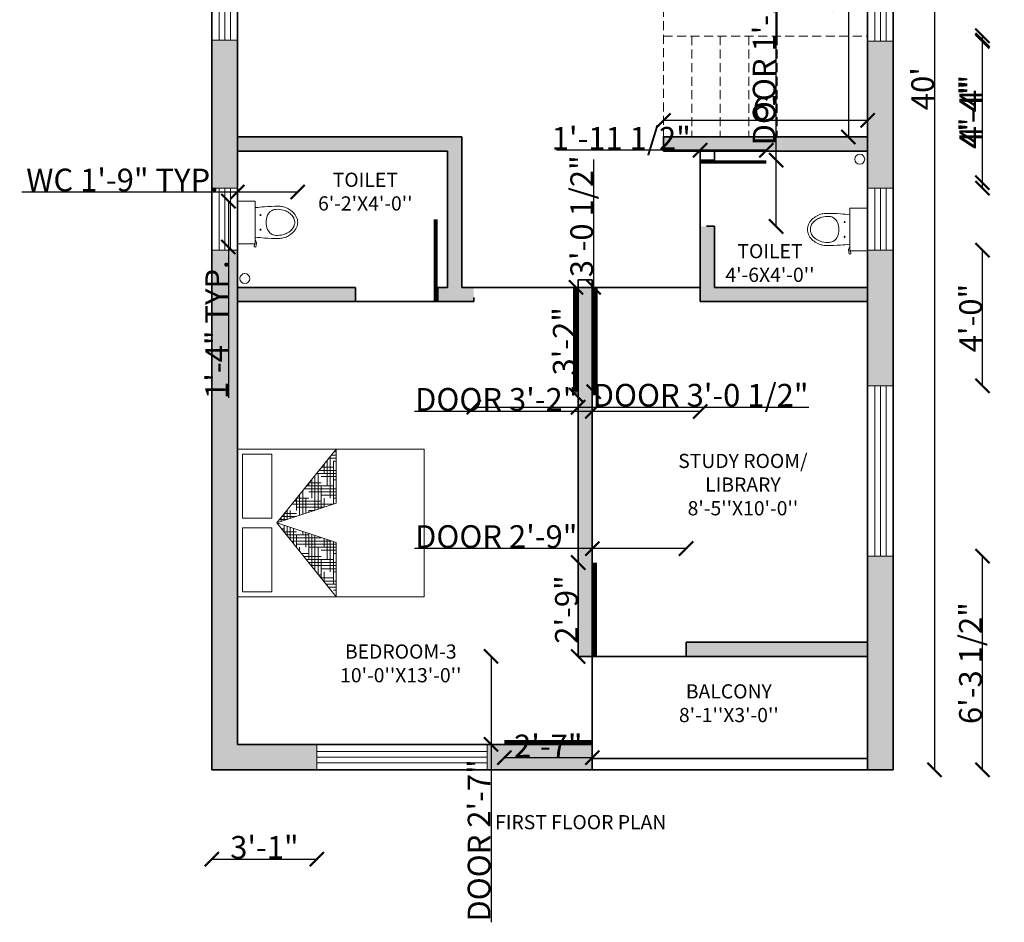
# Model space of a CAD drawing. Units: inches. Extents: x 2267 to 2908, y 1531 to 2136.
# Tile 4 of 5: x 2562 to 2908, y 1531 to 1849. Entities that reach past the tile are written whole.
import ezdxf

# ---------------------------------------------------------------- set-up
doc = ezdxf.new("R2010")
doc.units = ezdxf.units.IN
doc.linetypes.add('HIDDEN', pattern=[9.525, 6.35, -3.175])
for name, color, linetype, lineweight in [('A-ANNO-DIMS', 2, 'Continuous', 18), ('A-ANNO-TEXT', 7, 'Continuous', 18), ('A-AREA-IDEN', 7, 'Continuous', 18), ('A-FLOR-FIXT', 9, 'Continuous', 18), ('A-FLOR-STRS-HIDN', 50, 'HIDDEN', 13), ('A-FURN', 9, 'Continuous', 18), ('A-WALL-PATT', 8, 'Continuous', 13), ('DOOR', 30, 'Continuous', 18), ('STEPS', 50, 'Continuous', 18), ('WALL', 7, 'Continuous', 35), ('WINDOW', 152, 'Continuous', 18)]:
    doc.layers.add(name, color=color, linetype=linetype, lineweight=lineweight)
doc.styles.get("Standard").update_dxf_attribs({"font": 'arial.ttf'})
doc.dimstyles.get("Standard").update_dxf_attribs({"dimtxt": 8, "dimasz": 5, "dimexe": 0.18, "dimexo": 0.0625, "dimgap": 0.09, "dimtad": 1, "dimdec": 1, "dimzin": 0, "dimdsep": 46, "dimlunit": 4, "dimtxsty": 'Standard', "dimblk": 'ARCHTICK', "dimcen": 0.09, "dimse1": 1, "dimse2": 1, "dimadec": 0, "dimazin": 0, "dimtfac": 1, "dimtdec": 1, "dimtofl": 0, "dimtmove": 0, "dimatfit": 3, "dimfxl": 1, "dimtolj": 1, "dimtzin": 0, "dimarcsym": 0})

# ---------------------------------------------------------------- blocks, each defined once
blk = doc.blocks.new('A$C73484D89')
at = {"layer": 'DOOR'}
blk.add_lwpolyline([(1, 0, 0, 0, 0), (1, 0, 0, 0, 0), (0.975, 0, 0.05, 0.05, 0), (0.975, -1, 0, 0, 0), (0.95, -1, 0, 0, -0.429311), (0, 0, 0, 0, 0), (0, 0, 0, 0, 0)], format="xyseb", dxfattribs=at)
blk = doc.blocks.new('toilet-1')
at = {"color": 0, "linetype": 'ByBlock'}
for p, q in [((-0.23, -0.02), (-0.23, -0.212)), ((0.23, -0.02), (-0.23, -0.02)), ((0.23, -0.02), (0.23, -0.212)), ((-0.23, -0.212), (0.23, -0.212)), ((0.263, -0.2), (0.23, -0.204)), ((0.266, -0.219), (0.263, -0.2)), ((-0.089, -0.268), (-0.07, -0.268)), ((-0.079, -0.259), (-0.079, -0.278)), ((0.089, -0.268), (0.07, -0.268)), ((0.079, -0.259), (0.079, -0.278)), ((0.192, -0.214), (0.221, -0.225)), ((0.221, -0.225), (0.266, -0.219)), ((0, -0.638), (0, -0.638))]:
    blk.add_line(p, q, dxfattribs=at)
for centre, radius, start, end in [((1.737, -0.452), 1.911, 175.7698, 180.3758), ((3.527, -0.624), 3.709, 173.6925, 175.1593), ((-3.527, -0.624), 3.709, 4.8413, 6.3171), ((-1.737, -0.452), 1.911, 359.6242, 4.2302), ((-0.041, -0.44), 0.0996, 145.1497, 175.881), ((-0.031, -0.446), 0.111, 113.8997, 145.1485), ((0, -0.517), 0.188, 66.0939, 113.9061), ((0.031, -0.446), 0.111, 34.8515, 66.1003), ((0.041, -0.44), 0.0996, 4.119, 34.8503), ((0.035, -0.463), 0.209, 180.3747, 194.3375), ((0.055, -0.458), 0.23, 194.3353, 209.622), ((0.098, -0.45), 0.239, 175.8862, 195.5931), ((0.096, -0.45), 0.237, 195.5969, 209.3771), ((-0.096, -0.45), 0.237, 330.6229, 344.4031), ((-0.098, -0.45), 0.239, 344.4069, 4.1138), ((-0.055, -0.458), 0.23, 330.3788, 345.6655), ((-0.035, -0.463), 0.209, 345.6614, 359.6243), ((0.065, -0.452), 0.241, 209.6273, 224.5489), ((0.023, -0.491), 0.153, 209.3871, 226.5438), ((0.018, -0.499), 0.175, 224.552, 245.714), ((0.015, -0.5), 0.142, 226.5501, 246.5527), ((0, -0.535), 0.103, 246.5493, 270.0042), ((0, -0.535), 0.103, 269.9958, 293.4507), ((-0.015, -0.5), 0.142, 293.4473, 313.4499), ((-0.018, -0.499), 0.175, 294.2865, 315.4485), ((-0.023, -0.491), 0.153, 313.4562, 330.6129), ((-0.065, -0.452), 0.241, 315.4504, 330.372), ((0, -0.538), 0.132, 245.5845, 269.8782), ((0, -0.538), 0.132, 270.1216, 294.4153)]:
    blk.add_arc(centre, radius, start, end, dxfattribs=at)
blk = doc.blocks.new('*X6')
at = {"color": 0}
for p, q in [((20.156, 14.625), (20.156, 14.728)), ((20.174, 14.75), (20.277, 14.75)), ((20.188, 14.75), (20.188, 14.767)), ((20.199, 14.781), (20.277, 14.781)), ((20.25, 14.812), (20.277, 14.812)), ((20.25, 14.319), (20.25, 14.75)), ((20.094, 14.375), (20.094, 14.65)), ((20.098, 14.656), (20.125, 14.656)), ((20.124, 14.688), (20.25, 14.688)), ((20.125, 14.5), (20.125, 14.689)), ((20.149, 14.719), (20.277, 14.719)), ((19.998, 14.531), (20.277, 14.531)), ((20.023, 14.562), (20.277, 14.562)), ((20.031, 14.247), (20.031, 14.573)), ((20.062, 14.257), (20.062, 14.612)), ((20.125, 14.594), (20.277, 14.594)), ((20.219, 14.309), (20.219, 14.625)), ((20.25, 14.625), (20.277, 14.625)), ((19.922, 14.438), (20, 14.438)), ((19.948, 14.469), (20.125, 14.469)), ((19.973, 14.5), (20.25, 14.5)), ((20, 14.237), (20, 14.5)), ((20.188, 14.299), (20.188, 14.5)), ((20.25, 14.438), (20.277, 14.438)), ((19.844, 14.185), (19.844, 14.34)), ((19.875, 14.25), (19.875, 14.379)), ((19.875, 14.344), (20.277, 14.344)), ((19.906, 14.375), (19.906, 14.417)), ((19.969, 14.226), (19.969, 14.375)), ((20, 14.375), (20.277, 14.375)), ((20.125, 14.406), (20.277, 14.406)), ((20.156, 14.288), (20.156, 14.375)), ((19.772, 14.25), (20, 14.25)), ((19.781, 14.164), (19.781, 14.262)), ((19.797, 14.281), (20.125, 14.281)), ((19.812, 14.174), (19.812, 14.301)), ((19.822, 14.312), (20.229, 14.312)), ((19.938, 14.216), (19.938, 14.25)), ((19.721, 14.188), (19.75, 14.188)), ((19.746, 14.219), (19.875, 14.219)), ((19.75, 14.154), (19.75, 14.223)), ((19.702, 14.094), (19.779, 14.094)), ((19.719, 14.073), (19.719, 14.114)), ((19.727, 14.062), (19.873, 14.062)), ((19.75, 14.034), (19.75, 14.103)), ((19.752, 14.031), (19.875, 14.031)), ((19.781, 13.995), (19.781, 14.093)), ((19.812, 14), (19.812, 14.082)), ((19.906, 13.84), (19.906, 14.051)), ((19.938, 13.801), (19.938, 14.041)), ((19.969, 13.875), (19.969, 14.031)), ((19.827, 13.938), (20.25, 13.938)), ((19.875, 13.878), (19.875, 14)), ((19.875, 13.969), (20.156, 13.969)), ((20, 14), (20, 14.02)), ((20, 14), (20.061, 14)), ((20.062, 13.645), (20.062, 14)), ((20.094, 13.625), (20.094, 13.989)), ((20.125, 13.75), (20.125, 13.979)), ((20.156, 13.875), (20.156, 13.969)), ((20.25, 13.5), (20.25, 13.937)), ((19.853, 13.906), (20.125, 13.906)), ((19.878, 13.875), (20, 13.875)), ((20.031, 13.684), (20.031, 13.875)), ((20.125, 13.844), (20.277, 13.844)), ((20.219, 13.451), (20.219, 13.875)), ((20.25, 13.875), (20.277, 13.875)), ((19.953, 13.781), (20.277, 13.781)), ((19.978, 13.75), (20.25, 13.75)), ((20, 13.812), (20.277, 13.812)), ((20, 13.723), (20, 13.75)), ((20.188, 13.49), (20.188, 13.75)), ((20.003, 13.719), (20.125, 13.719)), ((20.125, 13.656), (20.277, 13.656)), ((20.25, 13.688), (20.277, 13.688)), ((20.079, 13.625), (20.277, 13.625)), ((20.104, 13.594), (20.277, 13.594)), ((20.129, 13.562), (20.25, 13.562)), ((20.156, 13.529), (20.156, 13.625)), ((20.205, 13.469), (20.277, 13.469)), ((20.23, 13.438), (20.277, 13.438)), ((20.25, 13.5), (20.277, 13.5)), ((20.255, 13.406), (20.277, 13.406))]:
    blk.add_line(p, q, dxfattribs=at)
blk = doc.blocks.new('MAT-P13')
for p, q in [((-0.75, 0), (0.75, 0)), ((-0.75, 0), (-0.75, -1.9)), ((0.75, 0), (0.75, -1.9)), ((-0.7, -0.05), (-0.7, -0.35)), ((-0.7, -0.05), (-0.05, -0.05)), ((-0.05, -0.35), (-0.05, -0.05)), ((0.05, -0.05), (0.7, -0.05)), ((0.05, -0.35), (0.05, -0.05)), ((0.7, -0.05), (0.7, -0.35)), ((-0.75, -1.003), (0, -0.4)), ((0, -0.4), (-0.75, -1.003)), ((-0.7, -0.35), (-0.05, -0.35)), ((0, -0.4), (-0.2, -1.003)), ((0, -0.4), (0.2, -1.003)), ((0, -0.4), (0.75, -1.003)), ((0.05, -0.35), (0.7, -0.35)), ((-0.75, -1.003), (-0.2, -1.003)), ((0.2, -1.003), (0.75, -1.003)), ((0.75, -1.9), (-0.75, -1.9))]:
    blk.add_line(p, q)
at = {"xscale": -1, "rotation": 90}
blk.add_blockref('*X6', (14.128, 19.274), dxfattribs=at)
blk = doc.blocks.new('_ArchTick')
at = {"color": 0, "linetype": 'ByBlock', "const_width": 0.15}
blk.add_lwpolyline([(-0.5, -0.5), (0.5, 0.5)], dxfattribs=at)
blk = doc.blocks.new('*D12')
at = {"layer": 'A-ANNO-DIMS', "color": 0, "lineweight": -2, "transparency": 16777216}
blk.add_line((2883.79, 2065.17), (2883.79, 1585.17), dxfattribs=at)
at = {"layer": 'Defpoints', "color": 0, "transparency": 16777216}
for p in [(2869.23, 2065.17), (2869.23, 1585.17), (2883.79, 1585.17)]:
    blk.add_point(p, dxfattribs=at)
at = {"layer": 'A-ANNO-DIMS', "color": 0, "lineweight": -2, "transparency": 16777216, "xscale": 5, "yscale": 5, "zscale": 5}
for p, rotation in [((2883.79, 2065.17), 90), ((2883.79, 1585.17), 270)]:
    blk.add_blockref('_ArchTick', p, dxfattribs=dict(at, rotation=rotation))
at = {"layer": 'A-ANNO-DIMS', "color": 0, "transparency": 16777216, "insert": (2879.62, 1825.17), "char_height": 8, "attachment_point": 5, "rotation": 90}
blk.add_mtext("\\A1;40'", dxfattribs=at)
blk = doc.blocks.new('*D14')
at = {"layer": 'A-ANNO-DIMS', "color": 0, "lineweight": -2, "transparency": 16777216}
blk.add_line((2853.44, 1919.17), (2853.44, 1808.17), dxfattribs=at)
at = {"layer": 'Defpoints', "color": 0, "transparency": 16777216}
for p in [(2860.23, 1919.17), (2853.44, 1808.17), (2860.23, 1808.17)]:
    blk.add_point(p, dxfattribs=at)
at = {"layer": 'A-ANNO-DIMS', "color": 0, "lineweight": -2, "transparency": 16777216, "xscale": 5, "yscale": 5, "zscale": 5}
for p, rotation in [((2853.44, 1919.17), 90), ((2853.44, 1808.17), 270)]:
    blk.add_blockref('_ArchTick', p, dxfattribs=dict(at, rotation=rotation))
at = {"layer": 'A-ANNO-DIMS', "color": 0, "transparency": 16777216, "insert": (2849.26, 1863.67), "char_height": 8, "attachment_point": 5, "rotation": 90}
blk.add_mtext('\\A1;9\'-3"', dxfattribs=at)
blk = doc.blocks.new('*D15')
at = {"layer": 'A-ANNO-DIMS', "color": 0, "lineweight": -2, "transparency": 16777216}
blk.add_line((2860.23, 1813.97), (2788.33, 1813.97), dxfattribs=at)
at = {"layer": 'Defpoints', "color": 0, "transparency": 16777216}
for p in [(2788.33, 1813.97), (2788.33, 1808.17), (2860.23, 1808.17)]:
    blk.add_point(p, dxfattribs=at)
at = {"layer": 'A-ANNO-DIMS', "color": 0, "lineweight": -2, "transparency": 16777216, "xscale": 5, "yscale": 5, "zscale": 5, "rotation": 180}
blk.add_blockref('_ArchTick', (2788.33, 1813.97), dxfattribs=at)
at = {"layer": 'A-ANNO-DIMS', "color": 0, "lineweight": -2, "transparency": 16777216, "xscale": 5, "yscale": 5, "zscale": 5}
blk.add_blockref('_ArchTick', (2860.23, 1813.97), dxfattribs=at)
at = {"layer": 'A-ANNO-DIMS', "color": 0, "transparency": 16777216, "insert": (2824.28, 1818.14), "char_height": 8, "attachment_point": 5}
blk.add_mtext("\\A1;6'", dxfattribs=at)
blk = doc.blocks.new('WIN-60IN')
for p, q in [((0, 6.5), (60, 6.5)), ((0, 4.5), (60, 4.5)), ((0, 2.5), (60, 2.5))]:
    blk.add_line(p, q)
blk.add_lwpolyline([(0, 9), (60, 9), (60, 0), (0, 0)], close=True)
blk = doc.blocks.new('WIN-43_65IN')
for p, q in [((2.5, 0), (2.5, 43.65)), ((4.5, 0), (4.5, 43.65)), ((6.5, 0), (6.5, 43.65))]:
    blk.add_line(p, q)
blk.add_lwpolyline([(0, 0), (0, 43.65), (9, 43.65), (9, 0)], close=True)
blk = doc.blocks.new('WIN-21_82IN')
for p, q in [((2.5, 0), (2.5, 21.82)), ((4.5, 0), (4.5, 21.82)), ((6.5, 0), (6.5, 21.82))]:
    blk.add_line(p, q)
blk.add_lwpolyline([(0, 0), (0, 21.82), (9, 21.82), (9, 0)], close=True)
blk = doc.blocks.new('*D29')
at = {"layer": 'A-ANNO-DIMS', "color": 0, "lineweight": -2, "transparency": 16777216}
for p, q in [((2763.23, 1711.47), (2700.55, 1711.47)), ((2801.24, 1711.47), (2763.23, 1711.47))]:
    blk.add_line(p, q, dxfattribs=at)
at = {"layer": 'Defpoints', "color": 0, "transparency": 16777216}
for p in [(2763.23, 1717.17), (2801.24, 1717.17), (2763.23, 1711.47)]:
    blk.add_point(p, dxfattribs=at)
at = {"layer": 'A-ANNO-DIMS', "color": 0, "lineweight": -2, "transparency": 16777216, "xscale": 5, "yscale": 5, "zscale": 5, "rotation": 180}
blk.add_blockref('_ArchTick', (2763.23, 1711.47), dxfattribs=at)
at = {"layer": 'A-ANNO-DIMS', "color": 0, "lineweight": -2, "transparency": 16777216, "xscale": 5, "yscale": 5, "zscale": 5}
blk.add_blockref('_ArchTick', (2801.24, 1711.47), dxfattribs=at)
at = {"layer": 'A-ANNO-DIMS', "color": 0, "transparency": 16777216, "insert": (2729.39, 1715.7), "char_height": 8, "attachment_point": 5}
blk.add_mtext('\\A1;DOOR 3\'-2"', dxfattribs=at)
blk = doc.blocks.new('*D30')
at = {"layer": 'A-ANNO-DIMS', "color": 0, "lineweight": -2, "transparency": 16777216}
blk.add_line((2757.53, 1717.17), (2757.53, 1755.17), dxfattribs=at)
at = {"layer": 'Defpoints', "color": 0, "transparency": 16777216}
for p in [(2757.53, 1755.17), (2763.23, 1755.17), (2763.23, 1717.17)]:
    blk.add_point(p, dxfattribs=at)
at = {"layer": 'A-ANNO-DIMS', "color": 0, "lineweight": -2, "transparency": 16777216, "xscale": 5, "yscale": 5, "zscale": 5}
for p, rotation in [((2757.53, 1755.17), 90), ((2757.53, 1717.17), 270)]:
    blk.add_blockref('_ArchTick', p, dxfattribs=dict(at, rotation=rotation))
at = {"layer": 'A-ANNO-DIMS', "color": 0, "transparency": 16777216, "insert": (2753.35, 1736.17), "char_height": 8, "attachment_point": 5, "rotation": 90}
blk.add_mtext('\\A1;3\'-2"', dxfattribs=at)
blk = doc.blocks.new('*D33')
at = {"layer": 'A-ANNO-DIMS', "color": 0, "lineweight": -2, "transparency": 16777216}
for p, q in [((2721.49, 1712.93), (2758.23, 1712.93)), ((2758.23, 1712.93), (2839.55, 1712.93))]:
    blk.add_line(p, q, dxfattribs=at)
at = {"layer": 'Defpoints', "color": 0, "transparency": 16777216}
for p in [(2721.49, 1718.44), (2758.23, 1718.44), (2758.23, 1712.93)]:
    blk.add_point(p, dxfattribs=at)
at = {"layer": 'A-ANNO-DIMS', "color": 0, "lineweight": -2, "transparency": 16777216, "xscale": 5, "yscale": 5, "zscale": 5, "rotation": 180}
blk.add_blockref('_ArchTick', (2721.49, 1712.93), dxfattribs=at)
at = {"layer": 'A-ANNO-DIMS', "color": 0, "lineweight": -2, "transparency": 16777216, "xscale": 5, "yscale": 5, "zscale": 5}
blk.add_blockref('_ArchTick', (2758.23, 1712.93), dxfattribs=at)
at = {"layer": 'A-ANNO-DIMS', "color": 0, "transparency": 16777216, "insert": (2801.39, 1717.16), "char_height": 8, "attachment_point": 5}
blk.add_mtext('\\A1;DOOR 3\'-0 1/2"', dxfattribs=at)
blk = doc.blocks.new('*D34')
at = {"layer": 'A-ANNO-DIMS', "color": 0, "lineweight": -2, "transparency": 16777216}
for p, q in [((2763.74, 1755.17), (2763.74, 1800.25)), ((2763.74, 1718.44), (2763.74, 1755.17))]:
    blk.add_line(p, q, dxfattribs=at)
at = {"layer": 'Defpoints', "color": 0, "transparency": 16777216}
for p in [(2758.23, 1755.17), (2763.74, 1755.17), (2758.23, 1718.44)]:
    blk.add_point(p, dxfattribs=at)
at = {"layer": 'A-ANNO-DIMS', "color": 0, "lineweight": -2, "transparency": 16777216, "xscale": 5, "yscale": 5, "zscale": 5}
for p, rotation in [((2763.74, 1755.17), 90), ((2763.74, 1718.44), 270)]:
    blk.add_blockref('_ArchTick', p, dxfattribs=dict(at, rotation=rotation))
at = {"layer": 'A-ANNO-DIMS', "color": 0, "transparency": 16777216, "insert": (2759.51, 1780.21), "char_height": 8, "attachment_point": 5, "rotation": 90}
blk.add_mtext('\\A1;3\'-0 1/2"', dxfattribs=at)
blk = doc.blocks.new('*D35')
at = {"layer": 'A-ANNO-DIMS', "color": 0, "lineweight": -2, "transparency": 16777216}
for p, q in [((2828, 1799.95), (2828, 1887.49)), ((2828, 1776.66), (2828, 1799.95))]:
    blk.add_line(p, q, dxfattribs=at)
at = {"layer": 'Defpoints', "color": 0, "transparency": 16777216}
for p in [(2824.51, 1799.95), (2828, 1799.95), (2824.51, 1776.66)]:
    blk.add_point(p, dxfattribs=at)
at = {"layer": 'A-ANNO-DIMS', "color": 0, "lineweight": -2, "transparency": 16777216, "xscale": 5, "yscale": 5, "zscale": 5}
for p, rotation in [((2828, 1799.95), 90), ((2828, 1776.66), 270)]:
    blk.add_blockref('_ArchTick', p, dxfattribs=dict(at, rotation=rotation))
at = {"layer": 'A-ANNO-DIMS', "color": 0, "transparency": 16777216, "insert": (2823.77, 1846.22), "char_height": 8, "attachment_point": 5, "rotation": 90}
blk.add_mtext('\\A1;DOOR 1\'-11 1/2"', dxfattribs=at)
blk = doc.blocks.new('*D36')
at = {"layer": 'A-ANNO-DIMS', "color": 0, "lineweight": -2, "transparency": 16777216}
for p, q in [((2801.23, 1803.44), (2750.68, 1803.44)), ((2824.51, 1803.44), (2801.23, 1803.44))]:
    blk.add_line(p, q, dxfattribs=at)
at = {"layer": 'Defpoints', "color": 0, "transparency": 16777216}
for p in [(2801.23, 1803.44), (2801.23, 1799.95), (2824.51, 1799.95)]:
    blk.add_point(p, dxfattribs=at)
at = {"layer": 'A-ANNO-DIMS', "color": 0, "lineweight": -2, "transparency": 16777216, "xscale": 5, "yscale": 5, "zscale": 5, "rotation": 180}
blk.add_blockref('_ArchTick', (2801.23, 1803.44), dxfattribs=at)
at = {"layer": 'A-ANNO-DIMS', "color": 0, "lineweight": -2, "transparency": 16777216, "xscale": 5, "yscale": 5, "zscale": 5}
blk.add_blockref('_ArchTick', (2824.51, 1803.44), dxfattribs=at)
at = {"layer": 'A-ANNO-DIMS', "color": 0, "transparency": 16777216, "insert": (2773.45, 1807.67), "char_height": 8, "attachment_point": 5}
blk.add_mtext('\\A1;1\'-11 1/2"', dxfattribs=at)
blk = doc.blocks.new('*D37')
at = {"layer": 'A-ANNO-DIMS', "color": 0, "lineweight": -2, "transparency": 16777216}
for p, q in [((2727.58, 1625.18), (2727.58, 1594.17)), ((2727.58, 1594.17), (2727.58, 1531.49))]:
    blk.add_line(p, q, dxfattribs=at)
at = {"layer": 'Defpoints', "color": 0, "transparency": 16777216}
for p in [(2732.23, 1625.18), (2727.58, 1594.17), (2732.23, 1594.17)]:
    blk.add_point(p, dxfattribs=at)
at = {"layer": 'A-ANNO-DIMS', "color": 0, "lineweight": -2, "transparency": 16777216, "xscale": 5, "yscale": 5, "zscale": 5}
for p, rotation in [((2727.58, 1625.18), 90), ((2727.58, 1594.17), 270)]:
    blk.add_blockref('_ArchTick', p, dxfattribs=dict(at, rotation=rotation))
at = {"layer": 'A-ANNO-DIMS', "color": 0, "transparency": 16777216, "insert": (2723.35, 1560.33), "char_height": 8, "attachment_point": 5, "rotation": 90}
blk.add_mtext('\\A1;DOOR 2\'-7"', dxfattribs=at)
blk = doc.blocks.new('*D38')
at = {"layer": 'A-ANNO-DIMS', "color": 0, "lineweight": -2, "transparency": 16777216}
blk.add_line((2732.23, 1589.52), (2763.23, 1589.52), dxfattribs=at)
at = {"layer": 'Defpoints', "color": 0, "transparency": 16777216}
for p in [(2732.23, 1594.17), (2763.23, 1594.17), (2763.23, 1589.52)]:
    blk.add_point(p, dxfattribs=at)
at = {"layer": 'A-ANNO-DIMS', "color": 0, "lineweight": -2, "transparency": 16777216, "xscale": 5, "yscale": 5, "zscale": 5, "rotation": 180}
blk.add_blockref('_ArchTick', (2732.23, 1589.52), dxfattribs=at)
at = {"layer": 'A-ANNO-DIMS', "color": 0, "lineweight": -2, "transparency": 16777216, "xscale": 5, "yscale": 5, "zscale": 5}
blk.add_blockref('_ArchTick', (2763.23, 1589.52), dxfattribs=at)
at = {"layer": 'A-ANNO-DIMS', "color": 0, "transparency": 16777216, "insert": (2747.73, 1593.63), "char_height": 8, "attachment_point": 5}
blk.add_mtext('\\A1;2\'-7"', dxfattribs=at)
blk = doc.blocks.new('*D39')
at = {"layer": 'A-ANNO-DIMS', "color": 0, "lineweight": -2, "transparency": 16777216}
for p, q in [((2763.23, 1663.15), (2700.55, 1663.15)), ((2796.26, 1663.15), (2763.23, 1663.15))]:
    blk.add_line(p, q, dxfattribs=at)
at = {"layer": 'Defpoints', "color": 0, "transparency": 16777216}
for p in [(2763.23, 1663.15), (2763.23, 1658.2), (2796.26, 1658.2)]:
    blk.add_point(p, dxfattribs=at)
at = {"layer": 'A-ANNO-DIMS', "color": 0, "lineweight": -2, "transparency": 16777216, "xscale": 5, "yscale": 5, "zscale": 5, "rotation": 180}
blk.add_blockref('_ArchTick', (2763.23, 1663.15), dxfattribs=at)
at = {"layer": 'A-ANNO-DIMS', "color": 0, "lineweight": -2, "transparency": 16777216, "xscale": 5, "yscale": 5, "zscale": 5}
blk.add_blockref('_ArchTick', (2796.26, 1663.15), dxfattribs=at)
at = {"layer": 'A-ANNO-DIMS', "color": 0, "transparency": 16777216, "insert": (2729.39, 1667.38), "char_height": 8, "attachment_point": 5}
blk.add_mtext('\\A1;DOOR 2\'-9"', dxfattribs=at)
blk = doc.blocks.new('*D40')
at = {"layer": 'A-ANNO-DIMS', "color": 0, "lineweight": -2, "transparency": 16777216}
blk.add_line((2758.27, 1658.2), (2758.27, 1625.17), dxfattribs=at)
at = {"layer": 'Defpoints', "color": 0, "transparency": 16777216}
for p in [(2763.23, 1658.2), (2758.27, 1625.17), (2763.23, 1625.17)]:
    blk.add_point(p, dxfattribs=at)
at = {"layer": 'A-ANNO-DIMS', "color": 0, "lineweight": -2, "transparency": 16777216, "xscale": 5, "yscale": 5, "zscale": 5}
for p, rotation in [((2758.27, 1658.2), 90), ((2758.27, 1625.17), 270)]:
    blk.add_blockref('_ArchTick', p, dxfattribs=dict(at, rotation=rotation))
at = {"layer": 'A-ANNO-DIMS', "color": 0, "transparency": 16777216, "insert": (2754.1, 1641.68), "char_height": 8, "attachment_point": 5, "rotation": 90}
blk.add_mtext('\\A1;2\'-9"', dxfattribs=at)
blk = doc.blocks.new('*D49')
at = {"layer": 'A-ANNO-DIMS', "color": 0, "lineweight": -2, "transparency": 16777216}
for p, q in [((2638.23, 1788.75), (2562.23, 1788.75)), ((2659.45, 1788.75), (2638.23, 1788.75))]:
    blk.add_line(p, q, dxfattribs=at)
at = {"layer": 'Defpoints', "color": 0, "transparency": 16777216}
for p in [(2638.23, 1788.75), (2638.23, 1785.57), (2659.45, 1785.57)]:
    blk.add_point(p, dxfattribs=at)
at = {"layer": 'A-ANNO-DIMS', "color": 0, "lineweight": -2, "transparency": 16777216, "xscale": 5, "yscale": 5, "zscale": 5, "rotation": 180}
blk.add_blockref('_ArchTick', (2638.23, 1788.75), dxfattribs=at)
at = {"layer": 'A-ANNO-DIMS', "color": 0, "lineweight": -2, "transparency": 16777216, "xscale": 5, "yscale": 5, "zscale": 5}
blk.add_blockref('_ArchTick', (2659.45, 1788.75), dxfattribs=at)
at = {"layer": 'A-ANNO-DIMS', "color": 0, "transparency": 16777216, "insert": (2597.73, 1792.98), "char_height": 8, "attachment_point": 5}
blk.add_mtext('\\A1;WC 1\'-9" TYP.', dxfattribs=at)
blk = doc.blocks.new('*D50')
at = {"layer": 'A-ANNO-DIMS', "color": 0, "lineweight": -2, "transparency": 16777216}
for p, q in [((2635.05, 1785.57), (2635.05, 1769.38)), ((2635.05, 1769.38), (2635.05, 1716.19))]:
    blk.add_line(p, q, dxfattribs=at)
at = {"layer": 'Defpoints', "color": 0, "transparency": 16777216}
for p in [(2638.23, 1785.57), (2635.05, 1769.38), (2638.23, 1769.38)]:
    blk.add_point(p, dxfattribs=at)
at = {"layer": 'A-ANNO-DIMS', "color": 0, "lineweight": -2, "transparency": 16777216, "xscale": 5, "yscale": 5, "zscale": 5}
for p, rotation in [((2635.05, 1785.57), 90), ((2635.05, 1769.38), 270)]:
    blk.add_blockref('_ArchTick', p, dxfattribs=dict(at, rotation=rotation))
at = {"layer": 'A-ANNO-DIMS', "color": 0, "transparency": 16777216, "insert": (2630.94, 1740.28), "char_height": 8, "attachment_point": 5, "rotation": 90}
blk.add_mtext('\\A1;1\'-4" TYP.', dxfattribs=at)
blk = doc.blocks.new('*D58')
at = {"layer": 'A-ANNO-DIMS', "color": 0, "lineweight": -2, "transparency": 16777216}
blk.add_line((2629.23, 1553.72), (2666.23, 1553.72), dxfattribs=at)
at = {"layer": 'Defpoints', "color": 0, "transparency": 16777216}
for p in [(2629.23, 1585.17), (2666.23, 1585.17), (2666.23, 1553.72)]:
    blk.add_point(p, dxfattribs=at)
at = {"layer": 'A-ANNO-DIMS', "color": 0, "lineweight": -2, "transparency": 16777216, "xscale": 5, "yscale": 5, "zscale": 5, "rotation": 180}
blk.add_blockref('_ArchTick', (2629.23, 1553.72), dxfattribs=at)
at = {"layer": 'A-ANNO-DIMS', "color": 0, "lineweight": -2, "transparency": 16777216, "xscale": 5, "yscale": 5, "zscale": 5}
blk.add_blockref('_ArchTick', (2666.23, 1553.72), dxfattribs=at)
at = {"layer": 'A-ANNO-DIMS', "color": 0, "transparency": 16777216, "insert": (2647.73, 1557.9), "char_height": 8, "attachment_point": 5}
blk.add_mtext('\\A1;3\'-1"', dxfattribs=at)
blk = doc.blocks.new('*D59')
at = {"layer": 'A-ANNO-DIMS', "color": 0, "lineweight": -2, "transparency": 16777216}
blk.add_line((2900.68, 1585.17), (2900.68, 1660.44), dxfattribs=at)
at = {"layer": 'Defpoints', "color": 0, "transparency": 16777216}
for p in [(2869.23, 1660.44), (2900.68, 1660.44), (2869.23, 1585.17)]:
    blk.add_point(p, dxfattribs=at)
at = {"layer": 'A-ANNO-DIMS', "color": 0, "lineweight": -2, "transparency": 16777216, "xscale": 5, "yscale": 5, "zscale": 5}
for p, rotation in [((2900.68, 1660.44), 90), ((2900.68, 1585.17), 270)]:
    blk.add_blockref('_ArchTick', p, dxfattribs=dict(at, rotation=rotation))
at = {"layer": 'A-ANNO-DIMS', "color": 0, "transparency": 16777216, "insert": (2896.45, 1622.8), "char_height": 8, "attachment_point": 5, "rotation": 90}
blk.add_mtext('\\A1;6\'-3 1/2"', dxfattribs=at)
blk = doc.blocks.new('*D66')
at = {"layer": 'A-ANNO-DIMS', "color": 0, "lineweight": -2, "transparency": 16777216}
blk.add_line((2900.678151, 1792.054206), (2900.678151, 1843.818992), dxfattribs=at)
at = {"layer": 'Defpoints', "color": 0, "transparency": 16777216}
for p in [(2547.807772, 1843.818992), (2900.678151, 1843.818992), (2547.807772, 1792.054206)]:
    blk.add_point(p, dxfattribs=at)
at = {"layer": 'A-ANNO-DIMS', "color": 0, "lineweight": -2, "transparency": 16777216, "xscale": 5, "yscale": 5, "zscale": 5}
for p, rotation in [((2900.678151, 1843.818992), 90), ((2900.678151, 1792.054206), 270)]:
    blk.add_blockref('_ArchTick', p, dxfattribs=dict(at, rotation=rotation))
at = {"layer": 'A-ANNO-DIMS', "color": 0, "transparency": 16777216, "insert": (2896.588151, 1817.936599), "char_height": 8, "attachment_point": 5, "rotation": 90}
blk.add_mtext('\\A1;4\'-4"', dxfattribs=at)
blk = doc.blocks.new('*D68')
at = {"layer": 'A-ANNO-DIMS', "color": 0, "lineweight": -2, "transparency": 16777216}
blk.add_line((2900.678151, 1790.119588), (2900.678151, 1842.237756), dxfattribs=at)
at = {"layer": 'Defpoints', "color": 0, "transparency": 16777216}
for p in [(2629.228151, 1842.237756), (2900.678151, 1842.237756), (2629.228151, 1790.119588)]:
    blk.add_point(p, dxfattribs=at)
at = {"layer": 'A-ANNO-DIMS', "color": 0, "lineweight": -2, "transparency": 16777216, "xscale": 5, "yscale": 5, "zscale": 5}
for p, rotation in [((2900.678151, 1842.237756), 90), ((2900.678151, 1790.119588), 270)]:
    blk.add_blockref('_ArchTick', p, dxfattribs=dict(at, rotation=rotation))
at = {"layer": 'A-ANNO-DIMS', "color": 0, "transparency": 16777216, "insert": (2896.588151, 1816.178672), "char_height": 8, "attachment_point": 5, "rotation": 90}
blk.add_mtext('\\A1;4\'-4"', dxfattribs=at)
blk = doc.blocks.new('*D69')
at = {"layer": 'A-ANNO-DIMS', "color": 0, "lineweight": -2, "transparency": 16777216}
blk.add_line((2900.68, 1720.44), (2900.68, 1768.26), dxfattribs=at)
at = {"layer": 'Defpoints', "color": 0, "transparency": 16777216}
for p in [(2869.23, 1768.26), (2900.68, 1768.26), (2869.23, 1720.44)]:
    blk.add_point(p, dxfattribs=at)
at = {"layer": 'A-ANNO-DIMS', "color": 0, "lineweight": -2, "transparency": 16777216, "xscale": 5, "yscale": 5, "zscale": 5}
for p, rotation in [((2900.68, 1768.26), 90), ((2900.68, 1720.44), 270)]:
    blk.add_blockref('_ArchTick', p, dxfattribs=dict(at, rotation=rotation))
at = {"layer": 'A-ANNO-DIMS', "color": 0, "transparency": 16777216, "insert": (2896.5, 1744.35), "char_height": 8, "attachment_point": 5, "rotation": 90}
blk.add_mtext('\\A1;4\'-0"', dxfattribs=at)
blk = doc.blocks.new('*D70')
at = {"layer": 'A-ANNO-DIMS', "color": 0, "lineweight": -2, "transparency": 16777216}
blk.add_line((2900.678151, 1790.083457), (2900.678151, 1841.848243), dxfattribs=at)
at = {"layer": 'Defpoints', "color": 0, "transparency": 16777216}
for p in [(2869.228151, 1841.848243), (2900.678151, 1841.848243), (2869.228151, 1790.083457)]:
    blk.add_point(p, dxfattribs=at)
at = {"layer": 'A-ANNO-DIMS', "color": 0, "lineweight": -2, "transparency": 16777216, "xscale": 5, "yscale": 5, "zscale": 5}
for p, rotation in [((2900.678151, 1841.848243), 90), ((2900.678151, 1790.083457), 270)]:
    blk.add_blockref('_ArchTick', p, dxfattribs=dict(at, rotation=rotation))
at = {"layer": 'A-ANNO-DIMS', "color": 0, "transparency": 16777216, "insert": (2896.588151, 1815.96585), "char_height": 8, "attachment_point": 5, "rotation": 90}
blk.add_mtext('\\A1;4\'-4"', dxfattribs=at)

msp = doc.modelspace()

# ---------------------------------------------------------------- hatches: boundary and pattern name
at = {"layer": 'A-WALL-PATT', "transparency": 33554585}
h = msp.add_hatch(color=256, dxfattribs=at)
h.dxf.hatch_style = 1
h.paths.add_polyline_path([(2547.81, 2067.14), (2395.31, 2067.14), (2395.31, 2058.14), (2413.81, 2058.14), (2538.81, 2058.14), (2538.81, 2022.14), (2547.81, 2022.14)])
h.paths.add_polyline_path([(2335.31, 2067.14), (2307.81, 2067.14), (2307.81, 1992.99), (2316.81, 1992.99), (2316.81, 2058.14), (2335.31, 2058.14)])
h.paths.add_polyline_path([(2316.81, 1949.34), (2307.81, 1949.34), (2307.81, 1886.58), (2316.81, 1886.58)])
h.paths.add_polyline_path([(2316.81, 1842.93), (2307.81, 1842.93), (2307.81, 1791.76), (2316.81, 1791.76)])
h.paths.add_polyline_path([(2316.81, 1769.93), (2307.81, 1769.93), (2307.81, 1695.97), (2316.81, 1695.97)])
h.paths.add_polyline_path([(2316.81, 1652.32), (2307.81, 1652.32), (2307.81, 1587.14), (2344.81, 1587.14), (2344.81, 1596.14), (2316.81, 1596.14)])
h.paths.add_polyline_path([(2441.81, 1715.23, -0.025641), (2438.4, 1715.23), (2436.81, 1715.23), (2436.81, 1596.14), (2404.81, 1596.14), (2404.81, 1587.14), (2441.81, 1587.14)])
h.paths.add_polyline_path([(2547.81, 1770.23), (2538.81, 1770.23), (2538.81, 1752.14), (2542.81, 1752.14), (2542.81, 1587.14), (2547.81, 1587.14)])
h.paths.add_polyline_path([(2547.81, 1843.82), (2538.81, 1843.82), (2538.81, 1792.05), (2547.81, 1792.05)])
h.paths.add_polyline_path([(2547.81, 1962.14), (2538.81, 1962.14), (2538.81, 1887.47), (2547.81, 1887.47)])
h.paths.add_polyline_path([(2638.23, 1962.08), (2629.23, 1962.08), (2629.23, 1885.88), (2638.23, 1885.88)])
h.paths.add_polyline_path([(2638.23, 2056.17), (2860.23, 2056.17), (2860.23, 2020.17), (2869.23, 2020.17), (2869.23, 2065.17), (2629.23, 2065.17), (2629.23, 2022.08), (2638.23, 2022.08)])
h.paths.add_polyline_path([(2869.23, 1960.17), (2860.23, 1960.17), (2860.23, 1885.5), (2869.23, 1885.5)])
h.paths.add_polyline_path([(2869.23, 1841.85), (2860.23, 1841.85), (2860.23, 1790.08), (2869.23, 1790.08)])
h.paths.add_polyline_path([(2869.23, 1768.26), (2860.23, 1768.26), (2860.23, 1768.05), (2860.23, 1720.44), (2869.23, 1720.44)])
h.paths.add_polyline_path([(2869.23, 1660.44), (2860.23, 1660.44), (2860.23, 1585.17), (2869.23, 1585.17)])
h.paths.add_polyline_path([(2763.23, 1594.17), (2726.23, 1594.17), (2726.23, 1585.17), (2763.23, 1585.17)])
h.paths.add_polyline_path([(2666.23, 1594.17), (2638.23, 1594.17), (2638.23, 1768.3), (2629.23, 1768.3), (2629.23, 1585.17), (2666.23, 1585.17)])
h.paths.add_polyline_path([(2638.23, 1842.24), (2629.23, 1842.24), (2629.23, 1790.12), (2638.23, 1790.12)])
h = msp.add_hatch(color=256, dxfattribs=at)
h.dxf.hatch_style = 1
h.paths.add_polyline_path([(2763.23, 1755.17), (2758.23, 1755.17), (2758.23, 1625.17), (2760.21, 1625.17, -0.025641), (2763.23, 1625.17)])
h.paths.add_polyline_path([(2638.23, 1750.17), (2679.86, 1750.17, -0.025641), (2679.86, 1752.99), (2679.86, 1755.17), (2638.23, 1755.17)])
h.paths.add_polyline_path([(2860.23, 1625.17), (2860.23, 1630.17), (2796.25, 1630.17), (2796.25, 1628.39, -0.025641), (2796.25, 1625.17)])
h.paths.add_polyline_path([(2730.26, 1919.17), (2745.45, 1919.17), (2745.45, 1924.17), (2740.23, 1924.17), (2740.23, 2056.17), (2735.23, 2056.17), (2735.23, 1924.17), (2730.26, 1924.17)])
h.paths.add_polyline_path([(2860.23, 1919.17), (2860.23, 1924.17), (2774.38, 1924.17), (2774.38, 1921.99, -0.025641), (2774.38, 1919.17)])
h.paths.add_polyline_path([(2638.23, 1919.17), (2701.33, 1919.17, -0.025641), (2701.33, 1921.99), (2701.33, 1924.17), (2638.23, 1924.17)])
h.paths.add_polyline_path([(2538.81, 1752.14), (2538.81, 1757.14), (2441.81, 1757.14), (2441.81, 1762.09), (2439.73, 1762.09, -0.025641), (2436.81, 1762.09), (2436.81, 1750.17), (2441.81, 1750.17), (2441.81, 1752.14)])
h.paths.add_polyline_path([(2436.81, 1810.14), (2436.81, 1792.08), (2441.81, 1792.08), (2441.81, 1805.14), (2538.81, 1805.14), (2538.81, 1810.14)])
h.paths.add_polyline_path([(2346.81, 1805.14), (2346.81, 1810.14), (2316.81, 1810.14), (2316.81, 1805.14)], flags=0)
h.paths.add_polyline_path([(2376.81, 1810.14), (2371.81, 1810.14), (2371.81, 1757.14), (2316.81, 1757.14), (2316.81, 1752.14), (2376.81, 1752.14)])
h.paths.add_polyline_path([(2374.47, 1921.14), (2374.47, 1926.14), (2316.81, 1926.14), (2316.81, 1921.14)])
h.paths.add_polyline_path([(2413.81, 1921.14), (2421.94, 1921.14), (2421.94, 1926.14), (2418.81, 1926.14), (2418.81, 2058.14), (2413.81, 2058.14)])
h.paths.add_polyline_path([(2316.81, 2022.14), (2316.81, 2017.14), (2381.27, 2017.14), (2381.27, 2022.14)])
h.paths.add_polyline_path([(2455.63, 1926.14), (2455.63, 1924.43, -0.025641), (2455.63, 1921.14), (2538.81, 1921.14), (2538.81, 1926.14)])
h = msp.add_hatch(color=256, dxfattribs=at)
h.dxf.hatch_style = 1
h.paths.add_polyline_path([(2717.23, 1808.17), (2638.23, 1808.17), (2638.23, 1803.17), (2712.23, 1803.17), (2712.23, 1755.17), (2708.79, 1755.17), (2708.79, 1750.17), (2721.5, 1750.17), (2721.5, 1751.59, -0.025641), (2721.5, 1755.17), (2717.23, 1755.17)])
h = msp.add_hatch(color=256, dxfattribs=at)
h.dxf.hatch_style = 1
h.paths.add_polyline_path([(2801.23, 1755.17, -0.025641), (2801.23, 1751.47), (2801.23, 1750.17), (2860.23, 1750.17), (2860.23, 1755.17), (2806.23, 1755.17), (2806.23, 1776.67), (2803.5, 1776.67, -0.025641), (2801.23, 1776.67)])
h.paths.add_polyline_path([(2788.33, 1808.17), (2788.33, 1803.17), (2860.23, 1803.17), (2860.23, 1808.17)])
h.paths.add_polyline_path([(2666.28, 1779.4), (2700.3, 1779.4), (2700.3, 1798.05), (2666.28, 1798.05)], flags=9)

# ---------------------------------------------------------------- linework, layer by layer
at = {"layer": 'A-FLOR-FIXT'}
for centre in [(2857.46, 1800.31), (2640.83, 1758.27)]:
    msp.add_circle(centre, 1.74, dxfattribs=at)
at = {"layer": 'A-FLOR-STRS-HIDN', "ltscale": 0.5}
for p, q in [((2788.33, 1853.67), (2788.33, 1808.17)), ((2788.33, 1843.67), (2860.23, 1843.67)), ((2798.33, 1843.67), (2798.33, 1808.17)), ((2808.33, 1843.67), (2808.33, 1808.17)), ((2818.33, 1843.67), (2818.33, 1808.17)), ((2828.33, 1843.67), (2828.33, 1808.17))]:
    msp.add_line(p, q, dxfattribs=at)
at = {"layer": 'STEPS'}
msp.add_line((2828.33, 1919.17), (2828.33, 1843.67), dxfattribs=at)
at = {"layer": 'WALL'}
for p, q in [((2629.23, 2065.17), (2629.23, 1585.17)), ((2869.23, 2065.17), (2869.23, 1585.17)), ((2638.23, 2056.17), (2638.23, 1594.17)), ((2860.23, 2056.17), (2860.23, 1585.17)), ((2638.23, 1808.17), (2717.23, 1808.17)), ((2717.23, 1808.17), (2717.23, 1755.17)), ((2788.33, 1808.17), (2788.33, 1803.17)), ((2788.33, 1808.17), (2860.23, 1808.17)), ((2638.23, 1803.17), (2712.23, 1803.17)), ((2712.23, 1803.17), (2712.23, 1755.17)), ((2788.33, 1803.17), (2860.23, 1803.17)), ((2801.23, 1803.17), (2801.23, 1755.17)), ((2806.23, 1803.17), (2806.23, 1799.95)), ((2801.23, 1799.95), (2806.23, 1799.95)), ((2803.5, 1776.67), (2806.23, 1776.67)), ((2806.23, 1776.67), (2806.23, 1755.17)), ((2638.23, 1755.17), (2679.86, 1755.17)), ((2679.86, 1755.17), (2679.86, 1752.99)), ((2708.79, 1755.17), (2708.79, 1750.17)), ((2708.79, 1755.17), (2712.23, 1755.17)), ((2717.23, 1755.17), (2801.23, 1755.17)), ((2758.23, 1757.78), (2758.23, 1625.17)), ((2758.23, 1757.78), (2763.23, 1757.78)), ((2763.23, 1757.78), (2763.23, 1585.17)), ((2801.23, 1751.6), (2801.23, 1755.17)), ((2806.23, 1755.17), (2860.23, 1755.17)), ((2679.86, 1752.99), (2679.86, 1750.17)), ((2638.23, 1750.17), (2721.5, 1750.17)), ((2721.5, 1751.59), (2721.5, 1750.17)), ((2801.23, 1751.47), (2801.23, 1750.17)), ((2801.23, 1750.17), (2860.23, 1750.17)), ((2796.25, 1630.17), (2860.23, 1630.17)), ((2796.25, 1630.17), (2796.25, 1628.39)), ((2796.25, 1628.39), (2796.25, 1625.17)), ((2758.23, 1625.17), (2763.23, 1625.17)), ((2763.23, 1625.17), (2860.23, 1625.17)), ((2638.23, 1594.17), (2763.23, 1594.17)), ((2763.23, 1589.17), (2860.23, 1589.17)), ((2629.23, 1585.17), (2869.23, 1585.17))]:
    msp.add_line(p, q, dxfattribs=at)

# ---------------------------------------------------------------- block references
at = {"layer": 'A-FLOR-FIXT', "yscale": 32.64243157977233, "zscale": 32.64243157977233}
for p, xscale, rotation in [((2637.58, 1778.06), -32.64243157977233, 90), ((2860.88, 1775.56), 32.64243157977233, 270)]:
    msp.add_blockref('toilet-1', p, dxfattribs=dict(at, xscale=xscale, rotation=rotation))
at = {"layer": 'A-FURN', "xscale": 34.62184577987068, "yscale": 34.62184577987068, "zscale": 34.62184577987068, "rotation": 90}
msp.add_blockref('MAT-P13', (2638.23, 1672.17), dxfattribs=at)
at = {"layer": 'DOOR'}
for p, xscale, yscale, zscale, rotation in [((2801.23, 1776.67), 23.27927248958356, 23.27927248958356, 23.27927248958356, 90.00000000000003), ((2679.86, 1750.17), -28.92760358030192, 28.92760358030192, 28.92760358030192, 180), ((2796.25, 1625.17), 33.02483188188864, 33.02483188188864, 33.02483188188864, 180), ((2763.23, 1625.17), 31.00000000000008, 31.00000000000008, 31.00000000000008, 270)]:
    msp.add_blockref('A$C73484D89', p, dxfattribs=dict(at, xscale=xscale, yscale=yscale, zscale=zscale, rotation=rotation))
for p, xscale, yscale, zscale in [((2721.5, 1755.17), 36.73126376560378, 36.73126376560378, 36.73126376560378), ((2801.23, 1755.17), -38.00000000000013, 38.00000000000013, 38.00000000000013)]:
    msp.add_blockref('A$C73484D89', p, dxfattribs=dict(at, xscale=xscale, yscale=yscale, zscale=zscale))
at = {"layer": 'WINDOW'}
for name, p in [('WIN-43_65IN', (2629.23, 1842.24)), ('WIN-43_65IN', (2860.23, 1841.85)), ('WIN-21_82IN', (2629.23, 1768.3)), ('WIN-21_82IN', (2860.23, 1768.26)), ('WIN-60IN', (2666.23, 1585.17))]:
    msp.add_blockref(name, p, dxfattribs=at)
at = {"layer": 'WINDOW', "rotation": 89.99999999999872}
msp.add_blockref('WIN-60IN', (2869.23, 1660.44), dxfattribs=at)

# ---------------------------------------------------------------- texts
at = {"layer": 'A-ANNO-TEXT', "insert": (2708.81, 1569.27), "char_height": 5, "attachment_point": 1}
msp.add_mtext_dynamic_manual_height_columns('\\pxqc;FIRST FLOOR PLAN', width=100.6772, gutter_width=12.5, heights=[0], dxfattribs=at)
at = {"layer": 'A-AREA-IDEN', "char_height": 5, "attachment_point": 1}
for s, width, insert in [("\\pxqc;TOILET\\P6'-2'X4'-0''", 41.4104, (2662.56, 1795.57)), ("\\pxqc;TOILET\\P4'-6X4'-0''", 41.4104, (2805.12, 1770.42)), ("\\pxqc;STUDY ROOM/\\PLIBRARY\\P8'-5''X10'-0''", 52.4916, (2790.05, 1696.52)), ("\\pxqc;BEDROOM-3\\P10'-0''X13'-0''", 41.4104, (2675.06, 1629.37)), ("\\pxqc;BALCONY\\P8'-1''X3'-0''", 41.4104, (2790.63, 1615.34))]:
    msp.add_mtext_dynamic_manual_height_columns(s, width=width, gutter_width=12.5, heights=[0], dxfattribs=dict(at, insert=insert))

# ---------------------------------------------------------------- dimensions: what is measured, and where the dimension line sits
at = {"layer": 'A-ANNO-DIMS'}
for base, p1, p2, angle, override, picture, middle in [((2883.79, 1585.17), (2869.23, 2065.17), (2869.23, 1585.17), 90, {"dimclrd": 0, "dimclre": 0, "dimclrt": 0}, '*D12', (2879.62, 1825.17)), ((2853.44, 1808.17), (2860.23, 1919.17), (2860.23, 1808.17), 90, {"dimclrd": 0, "dimclre": 0, "dimclrt": 0}, '*D14', (2849.26, 1863.67)), ((2900.68, 1843.82), (2547.81, 1792.05), (2547.81, 1843.82), 90, {"dimdec": 1, "dimlfac": 1, "dimrnd": 0, "dimzin": 1, "dimdsep": 46, "dimlunit": 4, "dimfrac": 2}, '*D66', (2896.59, 1817.94)), ((2900.68, 1842.24), (2629.23, 1790.12), (2629.23, 1842.24), 90, {"dimdec": 1, "dimlfac": 1, "dimrnd": 0, "dimzin": 1, "dimdsep": 46, "dimlunit": 4, "dimfrac": 2}, '*D68', (2896.59, 1816.18)), ((2900.68, 1841.85), (2869.23, 1790.08), (2869.23, 1841.85), 90, {"dimdec": 1, "dimlfac": 1, "dimrnd": 0, "dimzin": 1, "dimdsep": 46, "dimlunit": 4, "dimfrac": 2}, '*D70', (2896.59, 1815.97)), ((2801.23, 1803.44), (2824.51, 1799.95), (2801.23, 1799.95), 180, {"dimdec": 1, "dimlfac": 1, "dimrnd": 0, "dimzin": 1, "dimdsep": 46, "dimlunit": 4, "dimfrac": 2}, '*D36', (2773.45, 1807.67)), ((2763.74, 1755.17), (2758.23, 1718.44), (2758.23, 1755.17), 90, {"dimdec": 1, "dimlfac": 1, "dimrnd": 0, "dimzin": 1, "dimdsep": 46, "dimlunit": 4, "dimfrac": 2}, '*D34', (2759.51, 1780.21)), ((2900.68, 1768.26), (2869.23, 1720.44), (2869.23, 1768.26), 90, {"dimdec": 1, "dimlfac": 1, "dimrnd": 0, "dimzin": 1, "dimdsep": 46, "dimlunit": 4, "dimfrac": 2}, '*D69', (2896.5, 1744.35)), ((2757.53, 1755.17), (2763.23, 1717.17), (2763.23, 1755.17), 90, {"dimdec": 1, "dimlfac": 1, "dimrnd": 0, "dimzin": 1, "dimdsep": 46, "dimlunit": 4, "dimfrac": 2}, '*D30', (2753.35, 1736.17)), ((2900.68, 1660.44), (2869.23, 1585.17), (2869.23, 1660.44), 90, {"dimdec": 1, "dimlfac": 1, "dimrnd": 0, "dimzin": 1, "dimdsep": 46, "dimlunit": 4, "dimfrac": 2}, '*D59', (2896.45, 1622.8)), ((2758.27, 1625.17), (2763.23, 1658.2), (2763.23, 1625.17), 270, {"dimdec": 1, "dimlfac": 1, "dimrnd": 0, "dimzin": 1, "dimdsep": 46, "dimlunit": 4, "dimfrac": 2}, '*D40', (2754.1, 1641.68))]:
    dim = msp.add_linear_dim(base=base, p1=p1, p2=p2, angle=angle, dimstyle='Standard', override=override, dxfattribs=at)
    dim.commit()
    dim.dimension.update_dxf_attribs({"geometry": picture, "text_midpoint": middle})
for base, p1, p2, angle, text, picture, middle in [((2828, 1799.95), (2824.51, 1776.66), (2824.51, 1799.95), 90, 'DOOR <>', '*D35', (2823.77, 1846.22)), ((2638.23, 1788.75), (2659.45, 1785.57), (2638.23, 1785.57), 180, 'WC <> TYP.', '*D49', (2597.73, 1792.98)), ((2635.05, 1769.38), (2638.23, 1785.57), (2638.23, 1769.38), 270, '<> TYP.', '*D50', (2630.94, 1740.28)), ((2763.23, 1711.47), (2801.24, 1717.17), (2763.23, 1717.17), 180, 'DOOR <>', '*D29', (2729.39, 1715.7)), ((2763.23, 1663.15), (2796.26, 1658.2), (2763.23, 1658.2), 180, 'DOOR <>', '*D39', (2729.39, 1667.38)), ((2727.58, 1594.17), (2732.23, 1625.18), (2732.23, 1594.17), 270, 'DOOR <>', '*D37', (2723.35, 1560.33))]:
    dim = msp.add_linear_dim(base=base, p1=p1, p2=p2, angle=angle, text=text, dimstyle='Standard', override={"dimdec": 1, "dimlfac": 1, "dimrnd": 0, "dimzin": 1, "dimdsep": 46, "dimlunit": 4, "dimfrac": 2}, dxfattribs=at)
    dim.commit()
    dim.dimension.update_dxf_attribs({"geometry": picture, "text_midpoint": middle})
for base, p1, p2, override, picture, middle in [((2788.33, 1813.97), (2860.23, 1808.17), (2788.33, 1808.17), {"dimclrd": 0, "dimclre": 0, "dimclrt": 0}, '*D15', (2824.28, 1818.14)), ((2763.23, 1589.52), (2732.23, 1594.17), (2763.23, 1594.17), {"dimdec": 1, "dimlfac": 1, "dimrnd": 0, "dimzin": 1, "dimdsep": 46, "dimlunit": 4, "dimfrac": 2}, '*D38', (2747.73, 1593.63)), ((2666.23, 1553.72), (2629.23, 1585.17), (2666.23, 1585.17), {"dimdec": 1, "dimlfac": 1, "dimrnd": 0, "dimzin": 1, "dimdsep": 46, "dimlunit": 4, "dimfrac": 2}, '*D58', (2647.73, 1557.9))]:
    dim = msp.add_linear_dim(base=base, p1=p1, p2=p2, dimstyle='Standard', override=override, dxfattribs=at)
    dim.commit()
    dim.dimension.update_dxf_attribs({"geometry": picture, "text_midpoint": middle})
dim = msp.add_linear_dim(base=(2758.23, 1712.93), p1=(2721.49, 1718.44), p2=(2758.23, 1718.44), text='DOOR <>', dimstyle='Standard', override={"dimdec": 1, "dimlfac": 1, "dimrnd": 0, "dimzin": 1, "dimdsep": 46, "dimlunit": 4, "dimfrac": 2}, dxfattribs=at)
dim.commit()
dim.dimension.update_dxf_attribs({"geometry": '*D33', "text_midpoint": (2801.39, 1717.16)})

doc.saveas('drawing.dxf')
